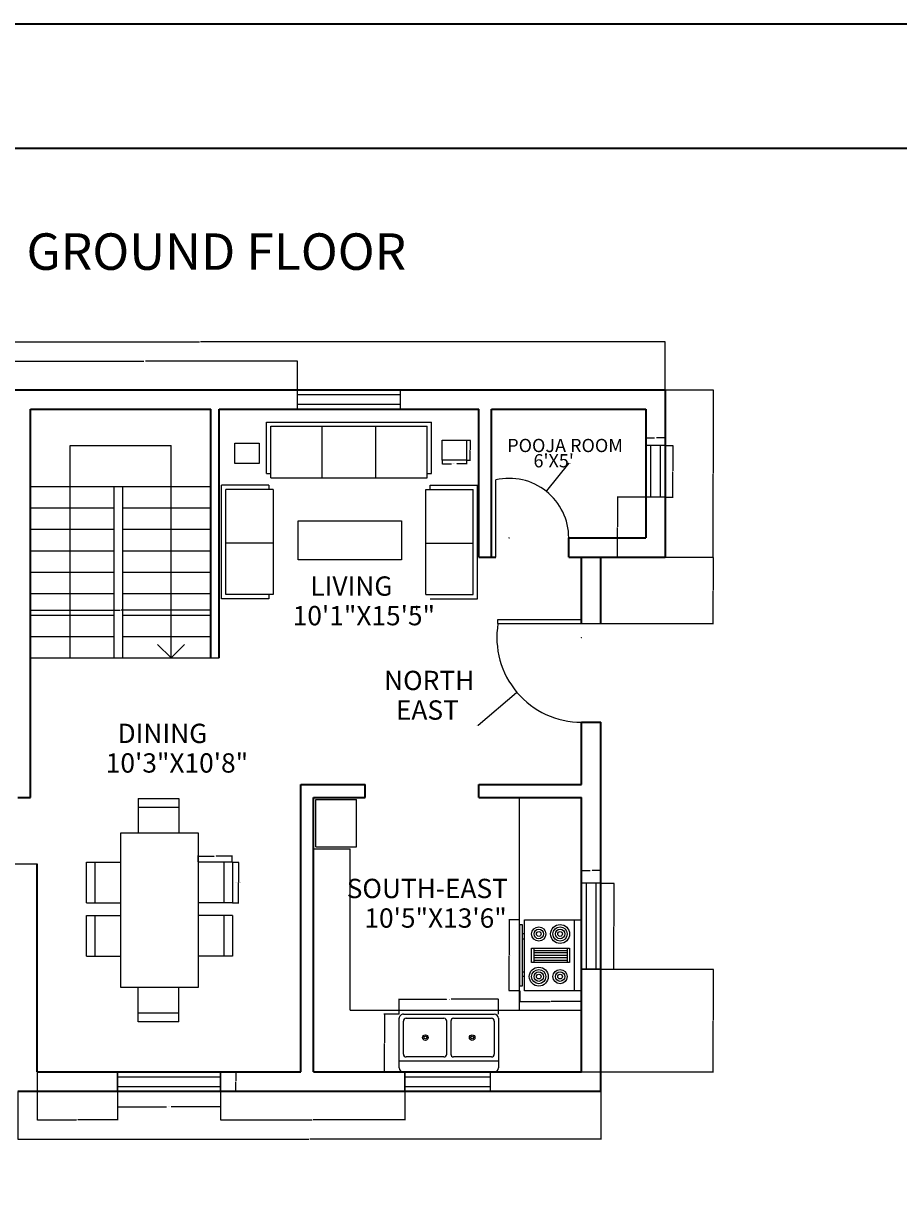
# Model space of a CAD drawing. Units: inches. Extents: x 2286 to 3750, y 1240 to 2345.
# Tile 5 of 7: x 2541 to 2949, y 1793 to 2345. Entities that reach past the tile are written whole.
import ezdxf

# ---------------------------------------------------------------- set-up
doc = ezdxf.new("R2010")
doc.units = ezdxf.units.IN
for name, color, linetype, lineweight in [('A-ANNO-DIMS', 2, 'Continuous', 18), ('A-ANNO-TEXT', 7, 'Continuous', 35), ('A-AREA-IDEN', 7, 'Continuous', 18), ('A-DOOR', 4, 'Continuous', 18), ('A-EQPM', 8, 'Continuous', 18), ('A-FLOR-CASE', 8, 'Continuous', 18), ('A-FLOR-FIXT', 9, 'Continuous', 18), ('A-FLOR-STRS', 7, 'Continuous', 18), ('A-FURN', 8, 'Continuous', 18), ('A-GLAZ', 51, 'Continuous', 18), ('A-WALL', 7, 'Continuous', 35)]:
    doc.layers.add(name, color=color, linetype=linetype, lineweight=lineweight)
doc.styles.get("Standard").update_dxf_attribs({"font": 'arial.ttf'})
doc.dimstyles.get("Standard").update_dxf_attribs({"dimtxt": 0.18, "dimasz": 0.18, "dimexe": 0.18, "dimexo": 0.0625, "dimgap": 0.09, "dimtad": 0, "dimtih": 1, "dimtoh": 1, "dimdec": 4, "dimzin": 0, "dimdsep": 46, "dimtxsty": 'Standard', "dimcen": 0.09, "dimadec": 0, "dimazin": 0, "dimtfac": 1, "dimtdec": 4, "dimtofl": 0, "dimtmove": 0, "dimatfit": 3, "dimfxl": 1, "dimtolj": 1, "dimtzin": 0, "dimarcsym": 0})

# ---------------------------------------------------------------- blocks, each defined once
blk = doc.blocks.new('Range-Oven - 30 in top')
for p, q in [((0, -3), (30, -3)), ((12, -6), (18, -6)), ((13, -20), (13, -6)), ((14, -6), (14, -20)), ((15, -20), (15, -6)), ((16, -6), (16, -20)), ((17, -20), (17, -6)), ((6, -24), (6, -25)), ((8, -25), (8, -24)), ((18, -20), (12, -20)), ((22, -25), (22, -24)), ((24, -24), (24, -25))]:
    blk.add_line(p, q)
for points in [[(0, -24), (0, 0), (30, 0), (30, -24)], [(12, -21), (12, -5), (18, -5), (18, -21)], [(2, -26), (2, -25), (28, -25), (28, -26)]]:
    blk.add_lwpolyline(points, close=True)
for centre, radius in [((6, -9), 4), ((6, -9), 3), ((6, -9), 2), ((6, -9), 1), ((24, -9), 3), ((24, -9), 2), ((24, -9), 1), ((24, -18), 4), ((6, -18), 3), ((6, -18), 2), ((6, -18), 1), ((24, -18), 3), ((24, -18), 2), ((24, -18), 1)]:
    blk.add_circle(centre, radius)
blk = doc.blocks.new('Sink-double - 36 in top')
for p, q in [((-18, -4), (18, -4)), ((-0.75, -18.5), (-0.75, -6.5)), ((0.75, -6.5), (0.75, -18.5))]:
    blk.add_line(p, q)
for points in [[(-16.5, 0), (16.5, 0)], [(-18, -19.5), (-18, -1.5)], [(18, -1.5), (18, -19.5)], [(-16.5, -18.5), (-16.5, -6.5)], [(-15.5, -5.5), (-1.75, -5.5)], [(1.75, -5.5), (15.5, -5.5)], [(16.5, -6.5), (16.5, -18.5)], [(16.5, -21), (-16.5, -21)], [(-1.75, -19.5), (-15.5, -19.5)], [(15.5, -19.5), (1.75, -19.5)]]:
    blk.add_lwpolyline(points)
for centre, radius in [((-8.5, -12.5), 1), ((-8.5, -12.5), 0.5), ((8.5, -12.5), 1), ((8.5, -12.5), 0.5)]:
    blk.add_circle(centre, radius)
for centre, radius, start, end in [((-16.5, -1.5), 1.5, 90, 180), ((16.5, -1.5), 1.5, 0, 90), ((-15.5, -6.5), 1, 90, 180), ((-1.75, -6.5), 1, 0, 90), ((1.75, -6.5), 1, 90, 180), ((15.5, -6.5), 1, 0, 90), ((-16.5, -19.5), 1.5, 180, 270), ((-15.5, -18.5), 1, 180, 270), ((-1.75, -18.5), 1, 270, 0), ((1.75, -18.5), 1, 180, 270), ((15.5, -18.5), 1, 270, 0), ((16.5, -19.5), 1.5, 270, 0)]:
    blk.add_arc(centre, radius, start, end)
blk = doc.blocks.new('CHAIR-DINING')
for p, q in [((0, 0), (0, 16)), ((19, 0), (19, 16)), ((19, 4), (0, 4)), ((19, 0), (0, 0))]:
    blk.add_line(p, q)
blk = doc.blocks.new('WIN-48x9')
for p, q in [((0, 0), (0, 9)), ((0, 6.75), (48, 6.75)), ((48, 0), (48, 9)), ((0, 2.25), (48, 2.25))]:
    blk.add_line(p, q)
blk = doc.blocks.new('WIN-40x9')
for p, q in [((0, 0), (0, 9)), ((0, 6.75), (40, 6.75)), ((40, 0), (40, 9)), ((0, 2.25), (40, 2.25))]:
    blk.add_line(p, q)
blk = doc.blocks.new('WIN-24x9')
for p, q in [((0, 0), (0, 9)), ((0, 6.75), (24, 6.75)), ((24, 0), (24, 9)), ((0, 2.25), (24, 2.25))]:
    blk.add_line(p, q)
blk = doc.blocks.new('TABLE-END')
blk.add_lwpolyline([(0, 9.41), (11.32, 9.41), (11.32, 0), (0, 0)], close=True)
blk = doc.blocks.new('*D26')
at = {"layer": 'A-ANNO-DIMS', "color": 0, "lineweight": -2, "transparency": 16777216}
for p, q in [((2638.81, 1954.02), (2641.78, 1954.02)), ((2641.6, 1953.84), (2641.6, 1944.7)), ((2641.6, 1935.2), (2641.6, 1944.33)), ((2638.81, 1935.02), (2641.78, 1935.02))]:
    blk.add_line(p, q, dxfattribs=at)
at = {"layer": 'A-ANNO-DIMS', "color": 0, "transparency": 16777216}
for points in [[(2641.57, 1953.84), (2641.63, 1953.84), (2641.6, 1954.02)], [(2641.57, 1935.2), (2641.63, 1935.2), (2641.6, 1935.02)]]:
    blk.add_solid(points, dxfattribs=at)
at = {"layer": 'Defpoints', "color": 0, "transparency": 16777216}
for p in [(2638.75, 1954.02), (2641.6, 1954.02), (2638.75, 1935.02)]:
    blk.add_point(p, dxfattribs=at)
at = {"layer": 'A-ANNO-DIMS', "color": 0, "transparency": 16777216, "insert": (2641.6, 1944.52), "char_height": 0.18, "attachment_point": 5}
blk.add_mtext('\\A1;DINING CHAIR 19 TYP.', dxfattribs=at)
blk = doc.blocks.new('*D27')
at = {"layer": 'A-ANNO-DIMS', "color": 0, "lineweight": -2, "transparency": 16777216}
for p, q in [((2622.75, 1954.08), (2622.75, 1957.05)), ((2622.93, 1956.87), (2630.23, 1956.87)), ((2638.57, 1956.87), (2631.27, 1956.87)), ((2638.75, 1954.08), (2638.75, 1957.05))]:
    blk.add_line(p, q, dxfattribs=at)
at = {"layer": 'A-ANNO-DIMS', "color": 0, "transparency": 16777216}
for points in [[(2622.93, 1956.9), (2622.93, 1956.84), (2622.75, 1956.87)], [(2638.57, 1956.9), (2638.57, 1956.84), (2638.75, 1956.87)]]:
    blk.add_solid(points, dxfattribs=at)
at = {"layer": 'Defpoints', "color": 0, "transparency": 16777216}
for p in [(2622.75, 1956.87), (2622.75, 1954.02), (2638.75, 1954.02)]:
    blk.add_point(p, dxfattribs=at)
at = {"layer": 'A-ANNO-DIMS', "color": 0, "transparency": 16777216, "insert": (2630.75, 1956.87), "char_height": 0.18, "attachment_point": 5}
blk.add_mtext('\\A1;16 TYP.', dxfattribs=at)
blk = doc.blocks.new('*D32')
at = {"layer": 'A-ANNO-DIMS', "color": 0, "lineweight": -2, "transparency": 16777216}
for p, q in [((2585.16, 1847.13), (2585.16, 1839.81)), ((2633.16, 1847.13), (2633.16, 1839.81)), ((2585.34, 1839.99), (2608.05, 1839.99)), ((2632.98, 1839.99), (2610.28, 1839.99))]:
    blk.add_line(p, q, dxfattribs=at)
at = {"layer": 'A-ANNO-DIMS', "color": 0, "transparency": 16777216}
for points in [[(2585.34, 1840.02), (2585.34, 1839.96), (2585.16, 1839.99)], [(2632.98, 1840.02), (2632.98, 1839.96), (2633.16, 1839.99)]]:
    blk.add_solid(points, dxfattribs=at)
at = {"layer": 'Defpoints', "color": 0, "transparency": 16777216}
for p in [(2585.16, 1847.19), (2633.16, 1847.19), (2633.16, 1839.99)]:
    blk.add_point(p, dxfattribs=at)
at = {"layer": 'A-ANNO-DIMS', "color": 0, "transparency": 16777216, "insert": (2609.16, 1839.99), "char_height": 0.18, "attachment_point": 5}
blk.add_mtext('\\A1;WINDOW 48 TYP.', dxfattribs=at)
blk = doc.blocks.new('*D33')
at = {"layer": 'A-ANNO-DIMS', "color": 0, "lineweight": -2, "transparency": 16777216}
for p, q in [((2633.23, 1856.19), (2640.54, 1856.19)), ((2640.36, 1856.01), (2640.36, 1851.87)), ((2640.36, 1847.37), (2640.36, 1851.51)), ((2633.23, 1847.19), (2640.54, 1847.19))]:
    blk.add_line(p, q, dxfattribs=at)
at = {"layer": 'A-ANNO-DIMS', "color": 0, "transparency": 16777216}
for points in [[(2640.33, 1856.01), (2640.39, 1856.01), (2640.36, 1856.19)], [(2640.33, 1847.37), (2640.39, 1847.37), (2640.36, 1847.19)]]:
    blk.add_solid(points, dxfattribs=at)
at = {"layer": 'Defpoints', "color": 0, "transparency": 16777216}
for p in [(2633.16, 1856.19), (2640.36, 1856.19), (2633.16, 1847.19)]:
    blk.add_point(p, dxfattribs=at)
at = {"layer": 'A-ANNO-DIMS', "color": 0, "transparency": 16777216, "insert": (2640.36, 1851.69), "char_height": 0.18, "attachment_point": 5}
blk.add_mtext('\\A1;9 TYP.', dxfattribs=at)
blk = doc.blocks.new('*D34')
at = {"layer": 'A-ANNO-DIMS', "color": 0, "lineweight": -2, "transparency": 16777216}
for p, q in [((2840.73, 2148.19), (2844.44, 2148.19)), ((2844.26, 2148.01), (2844.26, 2136.37)), ((2844.26, 2124.37), (2844.26, 2136.01)), ((2840.73, 2124.19), (2844.44, 2124.19))]:
    blk.add_line(p, q, dxfattribs=at)
at = {"layer": 'A-ANNO-DIMS', "color": 0, "transparency": 16777216}
for points in [[(2844.23, 2148.01), (2844.29, 2148.01), (2844.26, 2148.19)], [(2844.23, 2124.37), (2844.29, 2124.37), (2844.26, 2124.19)]]:
    blk.add_solid(points, dxfattribs=at)
at = {"layer": 'Defpoints', "color": 0, "transparency": 16777216}
for p in [(2840.66, 2148.19), (2844.26, 2148.19), (2840.66, 2124.19)]:
    blk.add_point(p, dxfattribs=at)
at = {"layer": 'A-ANNO-DIMS', "color": 0, "transparency": 16777216, "insert": (2844.26, 2136.19), "char_height": 0.18, "attachment_point": 5}
blk.add_mtext('\\A1;WINDOW 24 TYP.', dxfattribs=at)
blk = doc.blocks.new('*D35')
at = {"layer": 'A-ANNO-DIMS', "color": 0, "lineweight": -2, "transparency": 16777216}
for p, q in [((2831.66, 2148.25), (2831.66, 2151.97)), ((2831.84, 2151.79), (2835.71, 2151.79)), ((2840.48, 2151.79), (2836.62, 2151.79)), ((2840.66, 2148.25), (2840.66, 2151.97))]:
    blk.add_line(p, q, dxfattribs=at)
at = {"layer": 'A-ANNO-DIMS', "color": 0, "transparency": 16777216}
for points in [[(2831.84, 2151.82), (2831.84, 2151.76), (2831.66, 2151.79)], [(2840.48, 2151.82), (2840.48, 2151.76), (2840.66, 2151.79)]]:
    blk.add_solid(points, dxfattribs=at)
at = {"layer": 'Defpoints', "color": 0, "transparency": 16777216}
for p in [(2831.66, 2151.79), (2831.66, 2148.19), (2840.66, 2148.19)]:
    blk.add_point(p, dxfattribs=at)
at = {"layer": 'A-ANNO-DIMS', "color": 0, "transparency": 16777216, "insert": (2836.16, 2151.79), "char_height": 0.18, "attachment_point": 5}
blk.add_mtext('\\A1;9 TYP.', dxfattribs=at)
blk = doc.blocks.new('*D42')
at = {"layer": 'A-ANNO-DIMS', "color": 0, "lineweight": -2, "transparency": 16777216}
for p, q in [((2810.73, 1944.19), (2816.84, 1944.19)), ((2816.66, 1944.01), (2816.66, 1924.37)), ((2816.66, 1904.37), (2816.66, 1924.01)), ((2810.73, 1904.19), (2816.84, 1904.19))]:
    blk.add_line(p, q, dxfattribs=at)
at = {"layer": 'A-ANNO-DIMS', "color": 0, "transparency": 16777216}
for points in [[(2816.63, 1944.01), (2816.69, 1944.01), (2816.66, 1944.19)], [(2816.63, 1904.37), (2816.69, 1904.37), (2816.66, 1904.19)]]:
    blk.add_solid(points, dxfattribs=at)
at = {"layer": 'Defpoints', "color": 0, "transparency": 16777216}
for p in [(2810.66, 1944.19), (2816.66, 1944.19), (2810.66, 1904.19)]:
    blk.add_point(p, dxfattribs=at)
at = {"layer": 'A-ANNO-DIMS', "color": 0, "transparency": 16777216, "insert": (2816.66, 1924.19), "char_height": 0.18, "attachment_point": 5}
blk.add_mtext('\\A1;WINDOW 40 TYP.', dxfattribs=at)
blk = doc.blocks.new('*D43')
at = {"layer": 'A-ANNO-DIMS', "color": 0, "lineweight": -2, "transparency": 16777216}
for p, q in [((2801.66, 1944.25), (2801.66, 1950.37)), ((2801.84, 1950.19), (2805.71, 1950.19)), ((2810.48, 1950.19), (2806.62, 1950.19)), ((2810.66, 1944.25), (2810.66, 1950.37))]:
    blk.add_line(p, q, dxfattribs=at)
at = {"layer": 'A-ANNO-DIMS', "color": 0, "transparency": 16777216}
for points in [[(2801.84, 1950.22), (2801.84, 1950.16), (2801.66, 1950.19)], [(2810.48, 1950.22), (2810.48, 1950.16), (2810.66, 1950.19)]]:
    blk.add_solid(points, dxfattribs=at)
at = {"layer": 'Defpoints', "color": 0, "transparency": 16777216}
for p in [(2801.66, 1950.19), (2801.66, 1944.19), (2810.66, 1944.19)]:
    blk.add_point(p, dxfattribs=at)
at = {"layer": 'A-ANNO-DIMS', "color": 0, "transparency": 16777216, "insert": (2806.16, 1950.19), "char_height": 0.18, "attachment_point": 5}
blk.add_mtext('\\A1;9 TYP.', dxfattribs=at)
blk = doc.blocks.new('*D44')
at = {"layer": 'A-ANNO-DIMS', "color": 0, "lineweight": -2, "transparency": 16777216}
for p, q in [((2736.59, 2141.32), (2736.59, 2139.51)), ((2736.77, 2139.69), (2740.99, 2139.69)), ((2747.73, 2139.69), (2743.51, 2139.69)), ((2747.91, 2141.32), (2747.91, 2139.51))]:
    blk.add_line(p, q, dxfattribs=at)
at = {"layer": 'A-ANNO-DIMS', "color": 0, "transparency": 16777216}
for points in [[(2736.77, 2139.72), (2736.77, 2139.66), (2736.59, 2139.69)], [(2747.73, 2139.72), (2747.73, 2139.66), (2747.91, 2139.69)]]:
    blk.add_solid(points, dxfattribs=at)
at = {"layer": 'Defpoints', "color": 0, "transparency": 16777216}
for p in [(2736.59, 2141.39), (2747.91, 2141.39), (2747.91, 2139.69)]:
    blk.add_point(p, dxfattribs=at)
at = {"layer": 'A-ANNO-DIMS', "color": 0, "transparency": 16777216, "insert": (2742.25, 2139.69), "char_height": 0.18, "attachment_point": 5}
blk.add_mtext('\\A1;END TABLE 11 TYP.', dxfattribs=at)
blk = doc.blocks.new('*D45')
at = {"layer": 'A-ANNO-DIMS', "color": 0, "lineweight": -2, "transparency": 16777216}
for p, q in [((2747.98, 2150.8), (2749.79, 2150.8)), ((2749.61, 2150.62), (2749.61, 2146.27)), ((2749.61, 2141.57), (2749.61, 2145.91)), ((2747.98, 2141.39), (2749.79, 2141.39))]:
    blk.add_line(p, q, dxfattribs=at)
at = {"layer": 'A-ANNO-DIMS', "color": 0, "transparency": 16777216}
for points in [[(2749.58, 2150.62), (2749.64, 2150.62), (2749.61, 2150.8)], [(2749.58, 2141.57), (2749.64, 2141.57), (2749.61, 2141.39)]]:
    blk.add_solid(points, dxfattribs=at)
at = {"layer": 'Defpoints', "color": 0, "transparency": 16777216}
for p in [(2747.91, 2150.8), (2749.61, 2150.8), (2747.91, 2141.39)]:
    blk.add_point(p, dxfattribs=at)
at = {"layer": 'A-ANNO-DIMS', "color": 0, "transparency": 16777216, "insert": (2749.61, 2146.09), "char_height": 0.18, "attachment_point": 5}
blk.add_mtext('\\A1;9 TYP.', dxfattribs=at)
blk = doc.blocks.new('*D54')
at = {"layer": 'A-ANNO-DIMS', "color": 0, "lineweight": -2, "transparency": 16777216}
for p, q in [((2772.79, 1927.15), (2767.7, 1927.15)), ((2767.88, 1926.97), (2767.88, 1910.77)), ((2767.88, 1894.2), (2767.88, 1910.4)), ((2772.79, 1894.02), (2767.7, 1894.02))]:
    blk.add_line(p, q, dxfattribs=at)
at = {"layer": 'A-ANNO-DIMS', "color": 0, "transparency": 16777216}
for points in [[(2767.85, 1926.97), (2767.91, 1926.97), (2767.88, 1927.15)], [(2767.85, 1894.2), (2767.91, 1894.2), (2767.88, 1894.02)]]:
    blk.add_solid(points, dxfattribs=at)
at = {"layer": 'Defpoints', "color": 0, "transparency": 16777216}
for p in [(2772.85, 1927.15), (2767.88, 1894.02), (2772.85, 1894.02)]:
    blk.add_point(p, dxfattribs=at)
at = {"layer": 'A-ANNO-DIMS', "color": 0, "transparency": 16777216, "insert": (2767.88, 1910.58), "char_height": 0.18, "attachment_point": 5}
blk.add_mtext('\\A1;RANGE 33', dxfattribs=at)
blk = doc.blocks.new('*D55')
at = {"layer": 'A-ANNO-DIMS', "color": 0, "lineweight": -2, "transparency": 16777216}
for p, q in [((2772.85, 1893.95), (2772.85, 1888.86)), ((2773.03, 1889.04), (2786.99, 1889.04)), ((2801.39, 1889.04), (2787.43, 1889.04)), ((2801.57, 1893.95), (2801.57, 1888.86))]:
    blk.add_line(p, q, dxfattribs=at)
at = {"layer": 'A-ANNO-DIMS', "color": 0, "transparency": 16777216}
for points in [[(2773.03, 1889.07), (2773.03, 1889.01), (2772.85, 1889.04)], [(2801.39, 1889.07), (2801.39, 1889.01), (2801.57, 1889.04)]]:
    blk.add_solid(points, dxfattribs=at)
at = {"layer": 'Defpoints', "color": 0, "transparency": 16777216}
for p in [(2772.85, 1894.02), (2801.57, 1894.02), (2801.57, 1889.04)]:
    blk.add_point(p, dxfattribs=at)
at = {"layer": 'A-ANNO-DIMS', "color": 0, "transparency": 16777216, "insert": (2787.21, 1889.04), "char_height": 0.18, "attachment_point": 5}
blk.add_mtext('\\A1;29', dxfattribs=at)
blk = doc.blocks.new('*D56')
at = {"layer": 'A-ANNO-DIMS', "color": 0, "lineweight": -2, "transparency": 16777216}
for p, q in [((2716.59, 1883.19), (2716.59, 1890.25)), ((2716.77, 1890.07), (2738.61, 1890.07)), ((2762.65, 1890.07), (2740.8, 1890.07)), ((2762.83, 1883.19), (2762.83, 1890.25))]:
    blk.add_line(p, q, dxfattribs=at)
at = {"layer": 'A-ANNO-DIMS', "color": 0, "transparency": 16777216}
for points in [[(2716.77, 1890.1), (2716.77, 1890.04), (2716.59, 1890.07)], [(2762.65, 1890.1), (2762.65, 1890.04), (2762.83, 1890.07)]]:
    blk.add_solid(points, dxfattribs=at)
at = {"layer": 'Defpoints', "color": 0, "transparency": 16777216}
for p in [(2716.59, 1890.07), (2716.59, 1883.13), (2762.83, 1883.13)]:
    blk.add_point(p, dxfattribs=at)
at = {"layer": 'A-ANNO-DIMS', "color": 0, "transparency": 16777216, "insert": (2739.71, 1890.07), "char_height": 0.18, "attachment_point": 5}
blk.add_mtext('\\A1;DOUBLE SINK 46', dxfattribs=at)
blk = doc.blocks.new('*D57')
at = {"layer": 'A-ANNO-DIMS', "color": 0, "lineweight": -2, "transparency": 16777216}
for p, q in [((2716.52, 1883.13), (2709.47, 1883.13)), ((2709.65, 1882.95), (2709.65, 1869.82)), ((2709.65, 1856.34), (2709.65, 1869.46)), ((2716.52, 1856.16), (2709.47, 1856.16))]:
    blk.add_line(p, q, dxfattribs=at)
at = {"layer": 'A-ANNO-DIMS', "color": 0, "transparency": 16777216}
for points in [[(2709.62, 1882.95), (2709.68, 1882.95), (2709.65, 1883.13)], [(2709.62, 1856.34), (2709.68, 1856.34), (2709.65, 1856.16)]]:
    blk.add_solid(points, dxfattribs=at)
at = {"layer": 'Defpoints', "color": 0, "transparency": 16777216}
for p in [(2716.59, 1883.13), (2709.65, 1856.16), (2716.59, 1856.16)]:
    blk.add_point(p, dxfattribs=at)
at = {"layer": 'A-ANNO-DIMS', "color": 0, "transparency": 16777216, "insert": (2709.65, 1869.64), "char_height": 0.18, "attachment_point": 5}
blk.add_mtext('\\A1;27', dxfattribs=at)
blk = doc.blocks.new('*D58')
at = {"layer": 'A-ANNO-DIMS', "color": 0, "lineweight": -2, "transparency": 16777216}
for p, q in [((2406.66, 2174.25), (2406.66, 2196.67)), ((2406.84, 2196.49), (2623.37, 2196.49)), ((2840.48, 2196.49), (2623.96, 2196.49)), ((2840.66, 2174.25), (2840.66, 2196.67))]:
    blk.add_line(p, q, dxfattribs=at)
at = {"layer": 'A-ANNO-DIMS', "color": 0, "transparency": 16777216}
for points in [[(2406.84, 2196.52), (2406.84, 2196.46), (2406.66, 2196.49)], [(2840.48, 2196.52), (2840.48, 2196.46), (2840.66, 2196.49)]]:
    blk.add_solid(points, dxfattribs=at)
at = {"layer": 'Defpoints', "color": 0, "transparency": 16777216}
for p in [(2840.66, 2196.49), (2406.66, 2174.19), (2840.66, 2174.19)]:
    blk.add_point(p, dxfattribs=at)
at = {"layer": 'A-ANNO-DIMS', "color": 0, "transparency": 16777216, "insert": (2623.66, 2196.49), "char_height": 0.18, "attachment_point": 5}
blk.add_mtext('\\A1;434', dxfattribs=at)
blk = doc.blocks.new('*D61')
at = {"layer": 'A-ANNO-DIMS', "color": 0, "lineweight": -2, "transparency": 16777216}
for p, q in [((2538.66, 1847.13), (2538.66, 1824.71)), ((2810.66, 1847.13), (2810.66, 1824.71)), ((2538.84, 1824.89), (2674.37, 1824.89)), ((2810.48, 1824.89), (2674.95, 1824.89))]:
    blk.add_line(p, q, dxfattribs=at)
at = {"layer": 'A-ANNO-DIMS', "color": 0, "transparency": 16777216}
for points in [[(2538.84, 1824.92), (2538.84, 1824.86), (2538.66, 1824.89)], [(2810.48, 1824.92), (2810.48, 1824.86), (2810.66, 1824.89)]]:
    blk.add_solid(points, dxfattribs=at)
at = {"layer": 'Defpoints', "color": 0, "transparency": 16777216}
for p in [(2538.66, 1847.19), (2810.66, 1847.19), (2810.66, 1824.89)]:
    blk.add_point(p, dxfattribs=at)
at = {"layer": 'A-ANNO-DIMS', "color": 0, "transparency": 16777216, "insert": (2674.66, 1824.89), "char_height": 0.18, "attachment_point": 5}
blk.add_mtext('\\A1;272', dxfattribs=at)
blk = doc.blocks.new('*D62')
at = {"layer": 'A-ANNO-DIMS', "color": 0, "lineweight": -2, "transparency": 16777216}
for p, q in [((2840.73, 2174.19), (2863.14, 2174.19)), ((2862.96, 2174.01), (2862.96, 2135.37)), ((2862.96, 2096.37), (2862.96, 2135.01)), ((2840.73, 2096.19), (2863.14, 2096.19))]:
    blk.add_line(p, q, dxfattribs=at)
at = {"layer": 'A-ANNO-DIMS', "color": 0, "transparency": 16777216}
for points in [[(2862.93, 2174.01), (2862.99, 2174.01), (2862.96, 2174.19)], [(2862.93, 2096.37), (2862.99, 2096.37), (2862.96, 2096.19)]]:
    blk.add_solid(points, dxfattribs=at)
at = {"layer": 'Defpoints', "color": 0, "transparency": 16777216}
for p in [(2840.66, 2174.19), (2862.96, 2174.19), (2840.66, 2096.19)]:
    blk.add_point(p, dxfattribs=at)
at = {"layer": 'A-ANNO-DIMS', "color": 0, "transparency": 16777216, "insert": (2862.96, 2135.19), "char_height": 0.18, "attachment_point": 5}
blk.add_mtext('\\A1;78', dxfattribs=at)
blk = doc.blocks.new('*D64')
at = {"layer": 'A-ANNO-DIMS', "color": 0, "lineweight": -2, "transparency": 16777216}
for p, q in [((2544.66, 2049.25), (2544.66, 2071.67)), ((2544.84, 2071.49), (2586.44, 2071.49)), ((2628.48, 2071.49), (2586.88, 2071.49)), ((2628.66, 2049.25), (2628.66, 2071.67))]:
    blk.add_line(p, q, dxfattribs=at)
at = {"layer": 'A-ANNO-DIMS', "color": 0, "transparency": 16777216}
for points in [[(2544.84, 2071.52), (2544.84, 2071.46), (2544.66, 2071.49)], [(2628.48, 2071.52), (2628.48, 2071.46), (2628.66, 2071.49)]]:
    blk.add_solid(points, dxfattribs=at)
at = {"layer": 'Defpoints', "color": 0, "transparency": 16777216}
for p in [(2628.66, 2071.49), (2544.66, 2049.19), (2628.66, 2049.19)]:
    blk.add_point(p, dxfattribs=at)
at = {"layer": 'A-ANNO-DIMS', "color": 0, "transparency": 16777216, "insert": (2586.66, 2071.49), "char_height": 0.18, "attachment_point": 5}
blk.add_mtext('\\A1;84', dxfattribs=at)
blk = doc.blocks.new('*D65')
at = {"layer": 'A-ANNO-DIMS', "color": 0, "lineweight": -2, "transparency": 16777216}
for p, q in [((2810.73, 2096.19), (2863.14, 2096.19)), ((2862.96, 2096.01), (2862.96, 2080.87)), ((2862.96, 2065.37), (2862.96, 2080.51)), ((2810.73, 2065.19), (2863.14, 2065.19))]:
    blk.add_line(p, q, dxfattribs=at)
at = {"layer": 'A-ANNO-DIMS', "color": 0, "transparency": 16777216}
for points in [[(2862.93, 2096.01), (2862.99, 2096.01), (2862.96, 2096.19)], [(2862.93, 2065.37), (2862.99, 2065.37), (2862.96, 2065.19)]]:
    blk.add_solid(points, dxfattribs=at)
at = {"layer": 'Defpoints', "color": 0, "transparency": 16777216}
for p in [(2810.66, 2096.19), (2862.96, 2096.19), (2810.66, 2065.19)]:
    blk.add_point(p, dxfattribs=at)
at = {"layer": 'A-ANNO-DIMS', "color": 0, "transparency": 16777216, "insert": (2862.96, 2080.69), "char_height": 0.18, "attachment_point": 5}
blk.add_mtext('\\A1;31', dxfattribs=at)
blk = doc.blocks.new('*D67')
at = {"layer": 'A-ANNO-DIMS', "color": 0, "lineweight": -2, "transparency": 16777216}
for p, q in [((2526.66, 2165.25), (2526.66, 2187.67)), ((2526.84, 2187.49), (2597.53, 2187.49)), ((2668.98, 2187.49), (2598.3, 2187.49)), ((2669.16, 2165.25), (2669.16, 2187.67))]:
    blk.add_line(p, q, dxfattribs=at)
at = {"layer": 'A-ANNO-DIMS', "color": 0, "transparency": 16777216}
for points in [[(2526.84, 2187.52), (2526.84, 2187.46), (2526.66, 2187.49)], [(2668.98, 2187.52), (2668.98, 2187.46), (2669.16, 2187.49)]]:
    blk.add_solid(points, dxfattribs=at)
at = {"layer": 'Defpoints', "color": 0, "transparency": 16777216}
for p in [(2669.16, 2187.49), (2526.66, 2165.19), (2669.16, 2165.19)]:
    blk.add_point(p, dxfattribs=at)
at = {"layer": 'A-ANNO-DIMS', "color": 0, "transparency": 16777216, "insert": (2597.91, 2187.49), "char_height": 0.18, "attachment_point": 5}
blk.add_mtext('\\A1;142.5', dxfattribs=at)
blk = doc.blocks.new('*D70')
at = {"layer": 'A-ANNO-DIMS', "color": 0, "lineweight": -2, "transparency": 16777216}
for p, q in [((2547.66, 1856.13), (2547.66, 1833.71)), ((2585.16, 1856.13), (2585.16, 1833.71)), ((2547.84, 1833.89), (2566.09, 1833.89)), ((2584.98, 1833.89), (2566.74, 1833.89))]:
    blk.add_line(p, q, dxfattribs=at)
at = {"layer": 'A-ANNO-DIMS', "color": 0, "transparency": 16777216}
for points in [[(2547.84, 1833.92), (2547.84, 1833.86), (2547.66, 1833.89)], [(2584.98, 1833.92), (2584.98, 1833.86), (2585.16, 1833.89)]]:
    blk.add_solid(points, dxfattribs=at)
at = {"layer": 'Defpoints', "color": 0, "transparency": 16777216}
for p in [(2547.66, 1856.19), (2585.16, 1856.19), (2547.66, 1833.89)]:
    blk.add_point(p, dxfattribs=at)
at = {"layer": 'A-ANNO-DIMS', "color": 0, "transparency": 16777216, "insert": (2566.41, 1833.89), "char_height": 0.18, "attachment_point": 5}
blk.add_mtext('\\A1;37.5', dxfattribs=at)
blk = doc.blocks.new('*D71')
at = {"layer": 'A-ANNO-DIMS', "color": 0, "lineweight": -2, "transparency": 16777216}
for p, q in [((2633.16, 1856.13), (2633.16, 1833.71)), ((2719.16, 1856.13), (2719.16, 1833.71)), ((2633.34, 1833.89), (2675.94, 1833.89)), ((2718.98, 1833.89), (2676.38, 1833.89))]:
    blk.add_line(p, q, dxfattribs=at)
at = {"layer": 'A-ANNO-DIMS', "color": 0, "transparency": 16777216}
for points in [[(2633.34, 1833.92), (2633.34, 1833.86), (2633.16, 1833.89)], [(2718.98, 1833.92), (2718.98, 1833.86), (2719.16, 1833.89)]]:
    blk.add_solid(points, dxfattribs=at)
at = {"layer": 'Defpoints', "color": 0, "transparency": 16777216}
for p in [(2633.16, 1856.19), (2719.16, 1856.19), (2633.16, 1833.89)]:
    blk.add_point(p, dxfattribs=at)
at = {"layer": 'A-ANNO-DIMS', "color": 0, "transparency": 16777216, "insert": (2676.16, 1833.89), "char_height": 0.18, "attachment_point": 5}
blk.add_mtext('\\A1;86', dxfattribs=at)
blk = doc.blocks.new('*D72')
at = {"layer": 'A-ANNO-DIMS', "color": 0, "lineweight": -2, "transparency": 16777216}
for p, q in [((2801.73, 1904.19), (2863.14, 1904.19)), ((2862.96, 1904.01), (2862.96, 1880.37)), ((2862.96, 1856.37), (2862.96, 1880.01)), ((2801.73, 1856.19), (2863.14, 1856.19))]:
    blk.add_line(p, q, dxfattribs=at)
at = {"layer": 'A-ANNO-DIMS', "color": 0, "transparency": 16777216}
for points in [[(2862.93, 1904.01), (2862.99, 1904.01), (2862.96, 1904.19)], [(2862.93, 1856.37), (2862.99, 1856.37), (2862.96, 1856.19)]]:
    blk.add_solid(points, dxfattribs=at)
at = {"layer": 'Defpoints', "color": 0, "transparency": 16777216}
for p in [(2801.66, 1904.19), (2862.96, 1904.19), (2801.66, 1856.19)]:
    blk.add_point(p, dxfattribs=at)
at = {"layer": 'A-ANNO-DIMS', "color": 0, "transparency": 16777216, "insert": (2862.96, 1880.19), "char_height": 0.18, "attachment_point": 5}
blk.add_mtext('\\A1;48', dxfattribs=at)
blk = doc.blocks.new('*D73')
at = {"layer": 'A-ANNO-DIMS', "color": 0, "lineweight": -2, "transparency": 16777216}
for p, q in [((2840.6, 2124.19), (2818.18, 2124.19)), ((2818.36, 2124.01), (2818.36, 2110.37)), ((2818.36, 2096.37), (2818.36, 2110.01)), ((2840.6, 2096.19), (2818.18, 2096.19))]:
    blk.add_line(p, q, dxfattribs=at)
at = {"layer": 'A-ANNO-DIMS', "color": 0, "transparency": 16777216}
for points in [[(2818.33, 2124.01), (2818.39, 2124.01), (2818.36, 2124.19)], [(2818.33, 2096.37), (2818.39, 2096.37), (2818.36, 2096.19)]]:
    blk.add_solid(points, dxfattribs=at)
at = {"layer": 'Defpoints', "color": 0, "transparency": 16777216}
for p in [(2818.36, 2124.19), (2840.66, 2124.19), (2840.66, 2096.19)]:
    blk.add_point(p, dxfattribs=at)
at = {"layer": 'A-ANNO-DIMS', "color": 0, "transparency": 16777216, "insert": (2818.36, 2110.19), "char_height": 0.18, "attachment_point": 5}
blk.add_mtext('\\A1;28', dxfattribs=at)
blk = doc.blocks.new('*D123')
at = {"layer": 'A-ANNO-DIMS', "color": 0, "lineweight": -2, "transparency": 16777216}
for p, q in [((2801.57, 2058.72), (2801.75, 2058.72)), ((2801.66, 2058.63), (2801.66, 2058.81)), ((2753.42, 2017.82), (2771.37, 2033.04)), ((2753.24, 2017.82), (2753.42, 2017.82))]:
    blk.add_line(p, q, dxfattribs=at)
at = {"layer": 'A-ANNO-DIMS', "color": 0, "transparency": 16777216}
blk.add_solid([(2771.35, 2033.06), (2771.39, 2033.02), (2771.51, 2033.16)], dxfattribs=at)
at = {"layer": 'Defpoints', "color": 0, "transparency": 16777216}
for p in [(2801.66, 2058.72), (2771.51, 2033.16)]:
    blk.add_point(p, dxfattribs=at)
at = {"layer": 'A-ANNO-DIMS', "color": 0, "transparency": 16777216, "insert": (2752.76, 2017.82), "char_height": 0.18, "attachment_point": 5}
blk.add_mtext('\\A1;R39.53', dxfattribs=at)
blk = doc.blocks.new('*D125')
at = {"layer": 'A-ANNO-DIMS', "color": 0, "lineweight": -2, "transparency": 16777216}
for p, q in [((2795.53, 2139.92), (2785.29, 2127.04)), ((2795.71, 2139.92), (2795.53, 2139.92)), ((2767.85, 2105.19), (2768.03, 2105.19)), ((2767.94, 2105.1), (2767.94, 2105.28))]:
    blk.add_line(p, q, dxfattribs=at)
at = {"layer": 'A-ANNO-DIMS', "color": 0, "transparency": 16777216}
blk.add_solid([(2785.27, 2127.06), (2785.32, 2127.02), (2785.18, 2126.9)], dxfattribs=at)
at = {"layer": 'Defpoints', "color": 0, "transparency": 16777216}
for p in [(2785.18, 2126.9), (2767.94, 2105.19)]:
    blk.add_point(p, dxfattribs=at)
at = {"layer": 'A-ANNO-DIMS', "color": 0, "transparency": 16777216, "insert": (2796.18, 2139.92), "char_height": 0.18, "attachment_point": 5}
blk.add_mtext('\\A1;R27.72', dxfattribs=at)

msp = doc.modelspace()

# ---------------------------------------------------------------- linework, layer by layer
at = {"layer": 'A-DOOR'}
for p, q in [((2761.6637, 2096.1892), (2761.6637, 2132.1892)), ((2762.6637, 2067.1892), (2801.6637, 2067.1892)), ((2762.6637, 2065.1892), (2762.6637, 2067.1892)), ((2762.6637, 2065.1892), (2810.6637, 2065.1892)), ((2505.6637, 1953.1892), (2547.6637, 1953.1892))]:
    msp.add_line(p, q, dxfattribs=at)
for centre, radius, start, end in [((2767.9431, 2105.1892), 27.7206, 360, 103.092582), ((2801.6637, 2058.7218), 39.5326, 170.584296, 270)]:
    msp.add_arc(centre, radius, start, end, dxfattribs=at)
at = {"layer": 'A-FLOR-CASE'}
for p, q in [((2677.6637, 1961.1892), (2677.6637, 1983.1892)), ((2677.6637, 1983.1892), (2696.6637, 1983.1892)), ((2696.6637, 1961.1892), (2696.6637, 1983.1892)), ((2772.6637, 1885.0773), (2772.6637, 1984.1892)), ((2677.6637, 1961.1892), (2696.6637, 1961.1892)), ((2676.6637, 1960.1892), (2693.6637, 1960.1892)), ((2693.6637, 1885.0773), (2693.6637, 1960.1892)), ((2693.6637, 1885.0773), (2801.6637, 1885.0773))]:
    msp.add_line(p, q, dxfattribs=at)
at = {"layer": 'A-FLOR-STRS'}
for p, q in [((2563.1637, 2049.1892), (2563.1637, 2148.1892)), ((2563.1637, 2148.1892), (2610.1637, 2148.1892)), ((2610.1637, 2049.1892), (2610.1637, 2148.1892)), ((2544.6637, 2129.1892), (2628.6637, 2129.1892)), ((2583.6637, 2049.1892), (2583.6637, 2129.1892)), ((2587.6637, 2049.1892), (2587.6637, 2129.1892)), ((2544.6637, 2119.1892), (2583.6637, 2119.1892)), ((2587.6637, 2119.1892), (2628.6637, 2119.1892)), ((2544.6637, 2109.1892), (2583.6637, 2109.1892)), ((2587.6637, 2109.1892), (2628.6637, 2109.1892)), ((2544.6637, 2099.1892), (2583.6637, 2099.1892)), ((2587.6637, 2099.1892), (2628.6637, 2099.1892)), ((2544.6637, 2089.1892), (2583.6637, 2089.1892)), ((2587.6637, 2089.1892), (2628.6637, 2089.1892)), ((2544.6637, 2079.1892), (2583.6637, 2079.1892)), ((2587.6637, 2079.1892), (2628.6637, 2079.1892)), ((2544.6637, 2069.1892), (2583.6637, 2069.1892)), ((2587.6637, 2069.1892), (2628.6637, 2069.1892)), ((2544.6637, 2059.1892), (2583.6637, 2059.1892)), ((2587.6637, 2059.1892), (2628.6637, 2059.1892)), ((2610.1637, 2049.1892), (2603.9127, 2055.4839)), ((2610.1637, 2049.1892), (2616.4146, 2055.4839)), ((2544.6637, 2049.1892), (2632.6637, 2049.1892))]:
    msp.add_line(p, q, dxfattribs=at)
at = {"layer": 'A-FURN'}
for p, q in [((2654.6637, 2159.1892), (2731.6637, 2159.1892)), ((2654.6637, 2135.1892), (2654.6637, 2159.1892)), ((2656.6637, 2157.1892), (2729.6637, 2157.1892)), ((2656.6637, 2133.1892), (2656.6637, 2157.1892)), ((2680.6437, 2133.1892), (2680.6437, 2157.1892)), ((2705.6837, 2133.1892), (2705.6837, 2157.1892)), ((2729.6637, 2133.1892), (2729.6637, 2157.1892)), ((2731.6637, 2135.1892), (2731.6637, 2159.1892)), ((2654.6637, 2135.1892), (2656.6637, 2135.1892)), ((2656.6637, 2133.1892), (2729.6637, 2133.1892)), ((2729.6637, 2135.1892), (2731.6637, 2135.1892)), ((2633.7349, 2076.754), (2633.7349, 2129.774)), ((2655.7349, 2129.774), (2633.7349, 2129.774)), ((2635.7349, 2078.754), (2635.7349, 2127.774)), ((2657.7349, 2127.774), (2635.7349, 2127.774)), ((2655.7349, 2129.774), (2655.7349, 2127.774)), ((2657.7349, 2127.774), (2657.7349, 2078.754)), ((2729.0764, 2078.754), (2729.0764, 2127.774)), ((2729.0764, 2078.754), (2729.0764, 2127.774)), ((2729.0764, 2127.774), (2751.0764, 2127.774)), ((2731.0764, 2129.774), (2753.0764, 2129.774)), ((2731.0764, 2127.774), (2731.0764, 2129.774)), ((2751.0764, 2078.754), (2751.0764, 2127.774)), ((2753.0764, 2076.754), (2753.0764, 2129.774)), ((2657.7349, 2102.734), (2635.7349, 2102.734)), ((2729.0764, 2102.734), (2751.0764, 2102.734)), ((2655.7349, 2076.754), (2633.7349, 2076.754)), ((2657.7349, 2078.754), (2635.7349, 2078.754)), ((2655.7349, 2078.754), (2655.7349, 2076.754)), ((2729.0764, 2078.754), (2751.0764, 2078.754)), ((2731.0764, 2076.754), (2753.0764, 2076.754)), ((2724.8823, 2071.4818), (2724.8823, 2073.4818)), ((2586.7515, 1967.6337), (2622.7515, 1967.6337)), ((2586.7515, 1895.6337), (2586.7515, 1967.6337)), ((2622.7515, 1967.6337), (2622.7515, 1895.6337)), ((2622.7515, 1895.6337), (2586.7515, 1895.6337))]:
    msp.add_line(p, q, dxfattribs=at)
msp.add_lwpolyline([(2669.4943, 2113.08), (2717.6395, 2113.08), (2717.6395, 2094.9139), (2669.4943, 2094.9139)], close=True, dxfattribs=at)
at = {"layer": 'A-WALL'}
for p, q in [((2406.6637, 2174.1892), (2840.6637, 2174.1892)), ((2840.6637, 2174.1892), (2840.6637, 2096.1892)), ((2544.6637, 1984.1892), (2544.6637, 2165.1892)), ((2544.6637, 2165.1892), (2628.6637, 2165.1892)), ((2628.6637, 2049.1892), (2628.6637, 2165.1892)), ((2632.6637, 2049.1892), (2632.6637, 2165.1892)), ((2632.6637, 2165.1892), (2753.6637, 2165.1892)), ((2753.6637, 2096.1892), (2753.6637, 2165.1892)), ((2759.6637, 2096.1892), (2759.6637, 2165.1892)), ((2759.6637, 2165.1892), (2831.6637, 2165.1892)), ((2831.6637, 2165.1892), (2831.6637, 2105.1892)), ((2795.6637, 2096.1892), (2795.6637, 2105.1892)), ((2795.6637, 2105.1892), (2831.6637, 2105.1892)), ((2753.6637, 2096.1892), (2759.6637, 2096.1892)), ((2753.6637, 2096.1892), (2761.6637, 2096.1892)), ((2795.6637, 2096.1892), (2840.6637, 2096.1892)), ((2795.6637, 2096.1892), (2801.6637, 2096.1892)), ((2801.6637, 2065.1892), (2801.6637, 2096.1892)), ((2810.6637, 2065.1892), (2810.6637, 2096.1892)), ((2801.6637, 2019.1892), (2810.6637, 2019.1892)), ((2801.6637, 1990.1892), (2801.6637, 2019.1892)), ((2810.6637, 1847.1892), (2810.6637, 2019.1892)), ((2670.6637, 1856.1892), (2670.6637, 1990.1892)), ((2670.6637, 1990.1892), (2700.6637, 1990.1892)), ((2700.6637, 1984.1892), (2700.6637, 1990.1892)), ((2753.6637, 1984.1892), (2753.6637, 1990.1892)), ((2753.6637, 1990.1892), (2801.6637, 1990.1892)), ((2538.6637, 1984.1892), (2544.6637, 1984.1892)), ((2676.6637, 1856.1892), (2676.6637, 1984.1892)), ((2676.6637, 1984.1892), (2700.6637, 1984.1892)), ((2753.6637, 1984.1892), (2801.6637, 1984.1892)), ((2801.6637, 1856.1892), (2801.6637, 1984.1892)), ((2547.6637, 1856.1892), (2547.6637, 1953.1892)), ((2547.6637, 1856.1892), (2670.6637, 1856.1892)), ((2676.6637, 1856.1892), (2801.6637, 1856.1892)), ((2538.6637, 1847.1892), (2810.6637, 1847.1892))]:
    msp.add_line(p, q, dxfattribs=at)
for points in [[(2286.2079, 2344.8717), (3750.2574, 2344.8717), (3750.2574, 1240.4105), (2286.2079, 1240.4105)], [(2354.794, 2286.8809), (3673.7575, 2286.8809), (3673.7575, 1335.3046), (2354.794, 1335.3046)]]:
    msp.add_lwpolyline(points, close=True, dxfattribs=at)

# ---------------------------------------------------------------- block references
at = {"layer": 'A-EQPM', "xscale": 1.104573532630865, "yscale": 1.104573532630865, "zscale": 1.104573532630865, "rotation": 270}
msp.add_blockref('Range-Oven - 30 in top', (2801.5666, 1927.1526), dxfattribs=at)
at = {"layer": 'A-FLOR-FIXT', "xscale": 1.284577568602302, "yscale": 1.284577568602302, "zscale": 1.284577568602302, "rotation": 180}
msp.add_blockref('Sink-double - 36 in top', (2739.708, 1856.1562), dxfattribs=at)
at = {"layer": 'A-FURN'}
for name, p in [('TABLE-END', (2639.9051, 2139.8752)), ('TABLE-END', (2736.59, 2141.3871)), ('CHAIR-DINING', (2594.7515, 1879.6337))]:
    msp.add_blockref(name, p, dxfattribs=at)
for p, rotation in [((2613.7515, 1983.6337), 180), ((2570.7515, 1954.0174), 270), ((2638.7515, 1935.0174), 90.00000000000003), ((2570.7515, 1929.1742), 270.0000000000007), ((2638.7515, 1910.1742), 89.9999999999993)]:
    msp.add_blockref('CHAIR-DINING', p, dxfattribs=dict(at, rotation=rotation))
at = {"layer": 'A-GLAZ'}
for name, p in [('WIN-48x9', (2669.1637, 2165.1892)), ('WIN-48x9', (2585.1637, 1847.1892)), ('WIN-40x9', (2719.1637, 1847.1892))]:
    msp.add_blockref(name, p, dxfattribs=at)
for name, p, rotation in [('WIN-24x9', (2840.6637, 2124.1892), 89.99999999999666), ('WIN-40x9', (2810.6637, 1904.1892), 89.99999999999841)]:
    msp.add_blockref(name, p, dxfattribs=dict(at, rotation=rotation))

# ---------------------------------------------------------------- texts
at = {"layer": 'A-ANNO-TEXT'}
msp.add_text('GROUND FLOOR', height=17, dxfattribs=at).set_placement((2542.7553, 2230.1297))
at = {"layer": 'A-AREA-IDEN'}
for s, height, p in [('POOJA ROOM', 6.16613, (2766.9693, 2145.1614)), ("      6'X5'", 6.166131, (2767.919, 2138.0439)), ('   LIVING', 9, (2666.9152, 2078.2144)), ('10\'1"X15\'5"', 9, (2666.9152, 2064.421)), ('NORTH', 9, (2709.5413, 2034.2127)), ('  EAST', 9, (2709.5413, 2020.4193)), ('  DINING', 9, (2579.7285, 2009.5404)), ('10\'3"X10\'8"', 9, (2579.7285, 1995.747)), ('SOUTH-EAST', 9, (2692.0982, 1937.2463)), ('   10\'5"X13\'6"', 9, (2692.0982, 1923.4529))]:
    msp.add_text(s, height=height, dxfattribs=at).set_placement(p)

# ---------------------------------------------------------------- dimensions: what is measured, and where the dimension line sits
at = {"layer": 'A-ANNO-DIMS'}
for base, p1, p2, picture, middle in [((2840.6637, 2196.4892), (2406.6637, 2174.1892), (2840.6637, 2174.1892), '*D58', (2623.6637, 2196.4892)), ((2628.6637, 2071.4892), (2544.6637, 2049.1892), (2628.6637, 2049.1892), '*D64', (2586.6637, 2071.4892)), ((2801.5666, 1889.0448), (2772.8477, 1894.0154), (2801.5666, 1894.0154), '*D55', (2787.2071, 1889.0448)), ((2810.6637, 1824.8892), (2538.6637, 1847.1892), (2810.6637, 1847.1892), '*D61', (2674.6637, 1824.8892))]:
    dim = msp.add_linear_dim(base=base, p1=p1, p2=p2, dimstyle='Standard', override={"dimdec": 0, "dimlfac": 1, "dimrnd": 0, "dimzin": 0, "dimdsep": 46, "dimlunit": 2}, dxfattribs=at)
    dim.commit()
    dim.dimension.update_dxf_attribs({"geometry": picture, "text_midpoint": middle})
for base, p1, p2, angle, override, picture, middle in [((2669.1637, 2187.4892), (2526.6637, 2165.1892), (2669.1637, 2165.1892), 0, {"dimdec": 1, "dimlfac": 1, "dimrnd": 0, "dimzin": 0, "dimdsep": 46, "dimlunit": 2}, '*D67', (2597.9137, 2187.4892)), ((2862.9637, 2174.1892), (2840.6637, 2096.1892), (2840.6637, 2174.1892), 90, {"dimdec": 0, "dimlfac": 1, "dimrnd": 0, "dimzin": 0, "dimdsep": 46, "dimlunit": 2}, '*D62', (2862.9637, 2135.1892)), ((2818.3637, 2124.1892), (2840.6637, 2096.1892), (2840.6637, 2124.1892), 90, {"dimdec": 0, "dimlfac": 1, "dimrnd": 0, "dimzin": 0, "dimdsep": 46, "dimlunit": 2}, '*D73', (2818.3637, 2110.1892)), ((2862.9637, 2096.1892), (2810.6637, 2065.1892), (2810.6637, 2096.1892), 90, {"dimdec": 0, "dimlfac": 1, "dimrnd": 0, "dimzin": 0, "dimdsep": 46, "dimlunit": 2}, '*D65', (2862.9637, 2080.6892)), ((2862.9637, 1904.1892), (2801.6637, 1856.1892), (2801.6637, 1904.1892), 90, {"dimdec": 0, "dimlfac": 1, "dimrnd": 0, "dimzin": 0, "dimdsep": 46, "dimlunit": 2}, '*D72', (2862.9637, 1880.1892)), ((2709.6489, 1856.1562), (2716.5856, 1883.1324), (2716.5856, 1856.1562), 270, {"dimdec": 0, "dimlfac": 1, "dimrnd": 0, "dimzin": 0, "dimdsep": 46, "dimlunit": 2}, '*D57', (2709.6489, 1869.6443)), ((2547.6637, 1833.8892), (2585.1637, 1856.1892), (2547.6637, 1856.1892), 180, {"dimdec": 1, "dimlfac": 1, "dimrnd": 0, "dimzin": 0, "dimdsep": 46, "dimlunit": 2}, '*D70', (2566.4137, 1833.8892)), ((2633.1637, 1833.8892), (2719.1637, 1856.1892), (2633.1637, 1856.1892), 180, {"dimdec": 0, "dimlfac": 1, "dimrnd": 0, "dimzin": 0, "dimdsep": 46, "dimlunit": 2}, '*D71', (2676.1637, 1833.8892))]:
    dim = msp.add_linear_dim(base=base, p1=p1, p2=p2, angle=angle, dimstyle='Standard', override=override, dxfattribs=at)
    dim.commit()
    dim.dimension.update_dxf_attribs({"geometry": picture, "text_midpoint": middle})
for base, p1, p2, angle, text, picture, middle in [((2749.6115, 2150.7982), (2747.913, 2141.3871), (2747.913, 2150.7982), 90, '<> TYP.', '*D45', (2749.6115, 2146.0927)), ((2831.6637, 2151.7892), (2840.6637, 2148.1892), (2831.6637, 2148.1892), 180, '<> TYP.', '*D35', (2836.1637, 2151.7892)), ((2844.2637, 2148.1892), (2840.6637, 2124.1892), (2840.6637, 2148.1892), 90, 'WINDOW <> TYP.', '*D34', (2844.2637, 2136.1892)), ((2622.7515, 1956.8674), (2638.7515, 1954.0174), (2622.7515, 1954.0174), 180, '<> TYP.', '*D27', (2630.7515, 1956.8674)), ((2641.6015, 1954.0174), (2638.7515, 1935.0174), (2638.7515, 1954.0174), 90, 'DINING CHAIR <> TYP.', '*D26', (2641.6015, 1944.5174)), ((2801.6637, 1950.1892), (2810.6637, 1944.1892), (2801.6637, 1944.1892), 180, '<> TYP.', '*D43', (2806.1637, 1950.1892)), ((2816.6637, 1944.1892), (2810.6637, 1904.1892), (2810.6637, 1944.1892), 90, 'WINDOW <> TYP.', '*D42', (2816.6637, 1924.1892)), ((2767.8771, 1894.0154), (2772.8477, 1927.1526), (2772.8477, 1894.0154), 270, 'RANGE <>', '*D54', (2767.8771, 1910.584)), ((2716.5856, 1890.0691), (2762.8304, 1883.1324), (2716.5856, 1883.1324), 180, 'DOUBLE SINK <>', '*D56', (2739.708, 1890.0691)), ((2640.3637, 1856.1892), (2633.1637, 1847.1892), (2633.1637, 1856.1892), 90, '<> TYP.', '*D33', (2640.3637, 1851.6892))]:
    dim = msp.add_linear_dim(base=base, p1=p1, p2=p2, angle=angle, text=text, dimstyle='Standard', override={"dimdec": 0, "dimlfac": 1, "dimrnd": 0, "dimzin": 0, "dimdsep": 46, "dimlunit": 2}, dxfattribs=at)
    dim.commit()
    dim.dimension.update_dxf_attribs({"geometry": picture, "text_midpoint": middle})
for base, p1, p2, text, picture, middle in [((2747.913, 2139.6886), (2736.59, 2141.3871), (2747.913, 2141.3871), 'END TABLE <> TYP.', '*D44', (2742.2515, 2139.6886)), ((2633.1637, 1839.9892), (2585.1637, 1847.1892), (2633.1637, 1847.1892), 'WINDOW <> TYP.', '*D32', (2609.1637, 1839.9892))]:
    dim = msp.add_linear_dim(base=base, p1=p1, p2=p2, text=text, dimstyle='Standard', override={"dimdec": 0, "dimlfac": 1, "dimrnd": 0, "dimzin": 0, "dimdsep": 46, "dimlunit": 2}, dxfattribs=at)
    dim.commit()
    dim.dimension.update_dxf_attribs({"geometry": picture, "text_midpoint": middle})
for center, mpoint, picture, middle in [((2767.9431, 2105.1892), (2785.1822, 2126.8973), '*D125', (2796.1847, 2139.9222)), ((2801.6637, 2058.7218), (2771.5098, 2033.1568), '*D123', (2752.7576, 2017.8178))]:
    dim = msp.add_radius_dim(center=center, mpoint=mpoint, dimstyle='Standard', override={"dimdec": 2, "dimlfac": 1, "dimrnd": 0, "dimzin": 0, "dimdsep": 46, "dimlunit": 2}, dxfattribs=at)
    dim.commit()
    dim.dimension.update_dxf_attribs({"geometry": picture, "text_midpoint": middle, "dimtype": 164})

doc.saveas('drawing.dxf')
